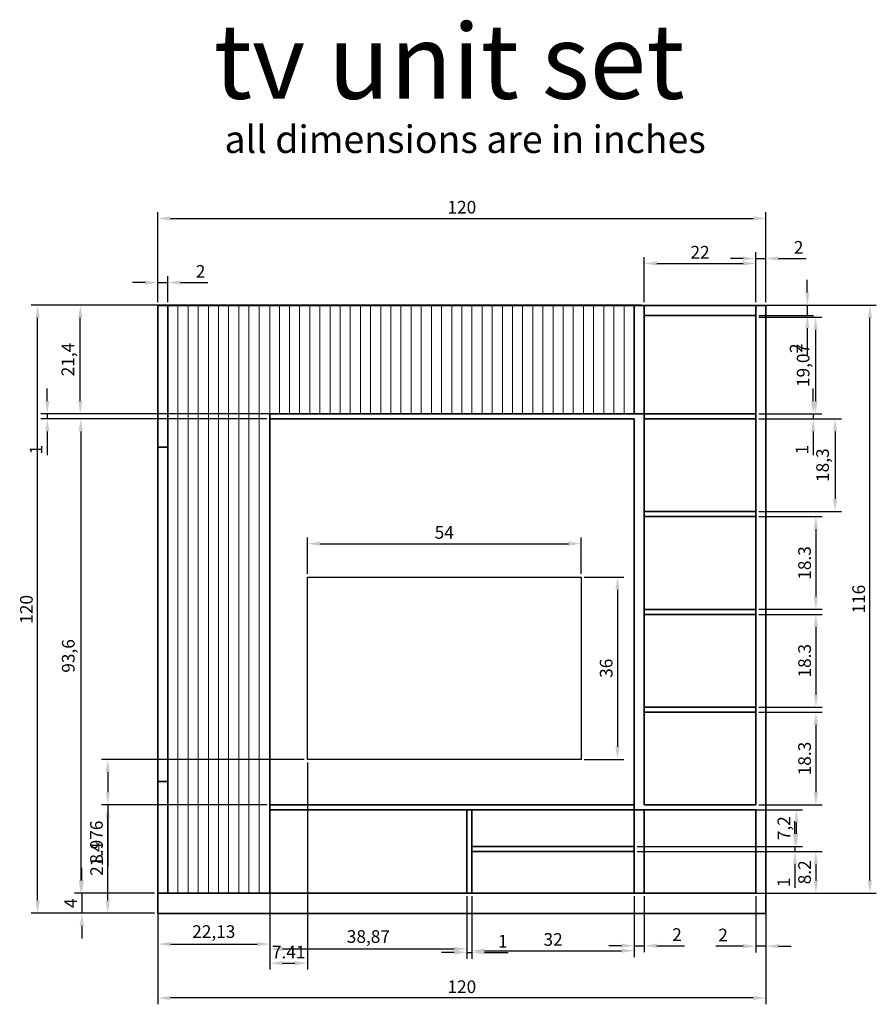
# Model space of a CAD drawing. Units: inches. Extents: x 64 to 1096, y 24 to 3074.
# Tile 1 of 1: x 64.3 to 233.3, y 23.5 to 217.9. Entities that reach past the tile are written whole.
import ezdxf

# ---------------------------------------------------------------- set-up
doc = ezdxf.new("R2010")
doc.units = ezdxf.units.IN
for name, color, linetype, lineweight in [('A-ANNO-DIMS', 2, 'Continuous', 18), ('A-ANNO-TEXT', 3, 'Continuous', 25), ('A-EQPM', 4, 'Continuous', 25), ('A-FURN', 7, 'Continuous', 35), ('A-FURN-PATT', 8, 'Continuous', 13)]:
    doc.layers.add(name, color=color, linetype=linetype, lineweight=lineweight)
doc.styles.get("Standard").update_dxf_attribs({"font": 'arial.ttf'})
doc.dimstyles.new('ISO-25', dxfattribs={"dimtxt": 2.5, "dimasz": 2.5, "dimexe": 1.25, "dimexo": 0.625, "dimtad": 1, "dimtxsty": 'Standard', "dimcen": 2.5, "dimadec": 0, "dimazin": 0, "dimtfac": 1, "dimtmove": 0, "dimatfit": 3, "dimfxl": 1, "dimarcsym": 0})

# ---------------------------------------------------------------- blocks, each defined once
blk = doc.blocks.new('*D1')
at = {"layer": 'A-ANNO-DIMS', "color": 0, "lineweight": -2, "transparency": 16777216}
for p, q in [((219.69, 163.98), (219.69, 166.48)), ((210.15, 161.48), (220.94, 161.48)), ((219.69, 161.48), (219.69, 159.48)), ((210.15, 159.48), (220.94, 159.48)), ((219.69, 156.98), (219.69, 151.57))]:
    blk.add_line(p, q, dxfattribs=at)
at = {"layer": 'A-ANNO-DIMS', "color": 0, "transparency": 16777216}
for points in [[(219.28, 163.98), (220.11, 163.98), (219.69, 161.48)], [(219.28, 156.98), (220.11, 156.98), (219.69, 159.48)]]:
    blk.add_solid(points, dxfattribs=at)
at = {"layer": 'Defpoints', "color": 0, "transparency": 16777216}
for p in [(209.53, 161.48), (209.53, 159.48), (219.69, 159.48)]:
    blk.add_point(p, dxfattribs=at)
at = {"layer": 'A-ANNO-DIMS', "color": 0, "transparency": 16777216, "insert": (217.81, 153.02), "char_height": 2.5, "attachment_point": 5, "rotation": 90}
blk.add_mtext('2', dxfattribs=at)
blk = doc.blocks.new('*D2')
at = {"layer": 'A-ANNO-DIMS', "color": 0, "lineweight": -2, "transparency": 16777216}
for p, q in [((210.15, 159.15), (222.57, 159.15)), ((221.32, 156.65), (221.32, 142.58)), ((210.15, 140.08), (222.57, 140.08))]:
    blk.add_line(p, q, dxfattribs=at)
at = {"layer": 'A-ANNO-DIMS', "color": 0, "transparency": 16777216}
for points in [[(220.9, 156.65), (221.73, 156.65), (221.32, 159.15)], [(220.9, 142.58), (221.73, 142.58), (221.32, 140.08)]]:
    blk.add_solid(points, dxfattribs=at)
at = {"layer": 'Defpoints', "color": 0, "transparency": 16777216}
for p in [(209.53, 159.15), (209.53, 140.08), (221.32, 140.08)]:
    blk.add_point(p, dxfattribs=at)
at = {"layer": 'A-ANNO-DIMS', "color": 0, "transparency": 16777216, "insert": (219.19, 149.61), "char_height": 2.5, "attachment_point": 5, "rotation": 90}
blk.add_mtext('19,07', dxfattribs=at)
blk = doc.blocks.new('*D3')
at = {"layer": 'A-ANNO-DIMS', "color": 0, "lineweight": -2, "transparency": 16777216}
for p, q in [((220.85, 142.58), (220.85, 145.08)), ((210.15, 140.08), (222.1, 140.08)), ((220.85, 140.08), (220.85, 139.08)), ((210.15, 139.08), (222.1, 139.08)), ((220.85, 136.58), (220.85, 131.91))]:
    blk.add_line(p, q, dxfattribs=at)
at = {"layer": 'A-ANNO-DIMS', "color": 0, "transparency": 16777216}
for points in [[(220.43, 142.58), (221.26, 142.58), (220.85, 140.08)], [(220.43, 136.58), (221.26, 136.58), (220.85, 139.08)]]:
    blk.add_solid(points, dxfattribs=at)
at = {"layer": 'Defpoints', "color": 0, "transparency": 16777216}
for p in [(209.53, 140.08), (209.53, 139.08), (220.85, 139.08)]:
    blk.add_point(p, dxfattribs=at)
at = {"layer": 'A-ANNO-DIMS', "color": 0, "transparency": 16777216, "insert": (218.97, 132.99), "char_height": 2.5, "attachment_point": 5, "rotation": 90}
blk.add_mtext('1', dxfattribs=at)
blk = doc.blocks.new('*D4')
at = {"layer": 'A-ANNO-DIMS', "color": 0, "lineweight": -2, "transparency": 16777216}
for p, q in [((210.15, 139.08), (226.41, 139.08)), ((225.16, 136.58), (225.16, 123.28)), ((210.15, 120.78), (226.41, 120.78))]:
    blk.add_line(p, q, dxfattribs=at)
at = {"layer": 'A-ANNO-DIMS', "color": 0, "transparency": 16777216}
for points in [[(224.74, 136.58), (225.58, 136.58), (225.16, 139.08)], [(224.74, 123.28), (225.58, 123.28), (225.16, 120.78)]]:
    blk.add_solid(points, dxfattribs=at)
at = {"layer": 'Defpoints', "color": 0, "transparency": 16777216}
for p in [(209.53, 139.08), (209.53, 120.78), (225.16, 120.78)]:
    blk.add_point(p, dxfattribs=at)
at = {"layer": 'A-ANNO-DIMS', "color": 0, "transparency": 16777216, "insert": (223.03, 129.93), "char_height": 2.5, "attachment_point": 5, "rotation": 90}
blk.add_mtext('18,3', dxfattribs=at)
blk = doc.blocks.new('*D5')
at = {"layer": 'A-ANNO-DIMS', "color": 0, "lineweight": -2, "transparency": 16777216}
for p, q in [((187.53, 162.1), (187.53, 171)), ((190.03, 169.75), (207.03, 169.75)), ((209.53, 162.1), (209.53, 171))]:
    blk.add_line(p, q, dxfattribs=at)
at = {"layer": 'A-ANNO-DIMS', "color": 0, "transparency": 16777216}
for points in [[(190.03, 170.17), (190.03, 169.33), (187.53, 169.75)], [(207.03, 170.17), (207.03, 169.33), (209.53, 169.75)]]:
    blk.add_solid(points, dxfattribs=at)
at = {"layer": 'Defpoints', "color": 0, "transparency": 16777216}
for p in [(209.53, 169.75), (187.53, 161.48), (209.53, 161.48)]:
    blk.add_point(p, dxfattribs=at)
at = {"layer": 'A-ANNO-DIMS', "color": 0, "transparency": 16777216, "insert": (198.53, 171.63), "char_height": 2.5, "attachment_point": 5}
blk.add_mtext('22', dxfattribs=at)
blk = doc.blocks.new('*D6')
at = {"layer": 'A-ANNO-DIMS', "color": 0, "lineweight": -2, "transparency": 16777216}
for p, q in [((209.53, 162.1), (209.53, 171.97)), ((211.53, 162.1), (211.53, 171.97)), ((207.03, 170.72), (204.53, 170.72)), ((209.53, 170.72), (211.53, 170.72)), ((214.03, 170.72), (219.43, 170.72))]:
    blk.add_line(p, q, dxfattribs=at)
at = {"layer": 'A-ANNO-DIMS', "color": 0, "transparency": 16777216}
for points in [[(207.03, 171.13), (207.03, 170.3), (209.53, 170.72)], [(214.03, 171.13), (214.03, 170.3), (211.53, 170.72)]]:
    blk.add_solid(points, dxfattribs=at)
at = {"layer": 'Defpoints', "color": 0, "transparency": 16777216}
for p in [(211.53, 170.72), (209.53, 161.48), (211.53, 161.48)]:
    blk.add_point(p, dxfattribs=at)
at = {"layer": 'A-ANNO-DIMS', "color": 0, "transparency": 16777216, "insert": (217.98, 172.6), "char_height": 2.5, "attachment_point": 5}
blk.add_mtext('2', dxfattribs=at)
blk = doc.blocks.new('*D7')
at = {"layer": 'A-ANNO-DIMS', "color": 0, "lineweight": -2, "transparency": 16777216}
for p, q in [((212.15, 161.48), (233.3, 161.48)), ((232.05, 47.98), (232.05, 158.98)), ((210.15, 45.48), (233.3, 45.48))]:
    blk.add_line(p, q, dxfattribs=at)
at = {"layer": 'A-ANNO-DIMS', "color": 0, "transparency": 16777216}
for points in [[(231.63, 158.98), (232.47, 158.98), (232.05, 161.48)], [(231.63, 47.98), (232.47, 47.98), (232.05, 45.48)]]:
    blk.add_solid(points, dxfattribs=at)
at = {"layer": 'Defpoints', "color": 0, "transparency": 16777216}
for p in [(211.53, 161.48), (232.05, 161.48), (209.53, 45.48)]:
    blk.add_point(p, dxfattribs=at)
at = {"layer": 'A-ANNO-DIMS', "color": 0, "transparency": 16777216, "insert": (230.15, 103.48), "char_height": 2.5, "attachment_point": 5, "rotation": 90}
blk.add_mtext('116', dxfattribs=at)
blk = doc.blocks.new('*D8')
at = {"layer": 'A-ANNO-DIMS', "color": 0, "lineweight": -2, "transparency": 16777216}
for p, q in [((91.53, 162.1), (91.53, 167.23)), ((93.53, 162.1), (93.53, 167.23)), ((89.03, 165.98), (86.53, 165.98)), ((91.53, 165.98), (93.53, 165.98)), ((96.03, 165.98), (101.43, 165.98))]:
    blk.add_line(p, q, dxfattribs=at)
at = {"layer": 'A-ANNO-DIMS', "color": 0, "transparency": 16777216}
for points in [[(89.03, 166.39), (89.03, 165.56), (91.53, 165.98)], [(96.03, 166.39), (96.03, 165.56), (93.53, 165.98)]]:
    blk.add_solid(points, dxfattribs=at)
at = {"layer": 'Defpoints', "color": 0, "transparency": 16777216}
for p in [(93.53, 165.98), (91.53, 161.48), (93.53, 161.48)]:
    blk.add_point(p, dxfattribs=at)
at = {"layer": 'A-ANNO-DIMS', "color": 0, "transparency": 16777216, "insert": (99.98, 167.86), "char_height": 2.5, "attachment_point": 5}
blk.add_mtext('2', dxfattribs=at)
blk = doc.blocks.new('*D9')
at = {"layer": 'A-ANNO-DIMS', "color": 0, "lineweight": -2, "transparency": 16777216}
for p, q in [((91.53, 162.1), (91.53, 179.88)), ((211.53, 162.1), (211.53, 179.88)), ((94.03, 178.63), (209.03, 178.63))]:
    blk.add_line(p, q, dxfattribs=at)
at = {"layer": 'A-ANNO-DIMS', "color": 0, "transparency": 16777216}
for points in [[(94.03, 179.05), (94.03, 178.21), (91.53, 178.63)], [(209.03, 179.05), (209.03, 178.21), (211.53, 178.63)]]:
    blk.add_solid(points, dxfattribs=at)
at = {"layer": 'Defpoints', "color": 0, "transparency": 16777216}
for p in [(211.53, 178.63), (91.53, 161.48), (211.53, 161.48)]:
    blk.add_point(p, dxfattribs=at)
at = {"layer": 'A-ANNO-DIMS', "color": 0, "transparency": 16777216, "insert": (151.53, 180.53), "char_height": 2.5, "attachment_point": 5}
blk.add_mtext('120', dxfattribs=at)
blk = doc.blocks.new('*D10')
at = {"layer": 'A-ANNO-DIMS', "color": 0, "lineweight": -2, "transparency": 16777216}
for p, q in [((186.9, 161.48), (75, 161.48)), ((76.25, 142.58), (76.25, 158.98)), ((186.9, 140.08), (75, 140.08))]:
    blk.add_line(p, q, dxfattribs=at)
at = {"layer": 'A-ANNO-DIMS', "color": 0, "transparency": 16777216}
for points in [[(75.83, 158.98), (76.66, 158.98), (76.25, 161.48)], [(75.83, 142.58), (76.66, 142.58), (76.25, 140.08)]]:
    blk.add_solid(points, dxfattribs=at)
at = {"layer": 'Defpoints', "color": 0, "transparency": 16777216}
for p in [(76.25, 161.48), (187.53, 161.48), (187.53, 140.08)]:
    blk.add_point(p, dxfattribs=at)
at = {"layer": 'A-ANNO-DIMS', "color": 0, "transparency": 16777216, "insert": (74.12, 150.78), "char_height": 2.5, "attachment_point": 5, "rotation": 90}
blk.add_mtext('21,4', dxfattribs=at)
blk = doc.blocks.new('*D11')
at = {"layer": 'A-ANNO-DIMS', "color": 0, "lineweight": -2, "transparency": 16777216}
for p, q in [((90.9, 139.08), (75.09, 139.08)), ((76.34, 136.58), (76.34, 47.98)), ((90.9, 45.48), (75.09, 45.48))]:
    blk.add_line(p, q, dxfattribs=at)
at = {"layer": 'A-ANNO-DIMS', "color": 0, "transparency": 16777216}
for points in [[(75.92, 136.58), (76.76, 136.58), (76.34, 139.08)], [(75.92, 47.98), (76.76, 47.98), (76.34, 45.48)]]:
    blk.add_solid(points, dxfattribs=at)
at = {"layer": 'Defpoints', "color": 0, "transparency": 16777216}
for p in [(91.53, 139.08), (76.34, 45.48), (91.53, 45.48)]:
    blk.add_point(p, dxfattribs=at)
at = {"layer": 'A-ANNO-DIMS', "color": 0, "transparency": 16777216, "insert": (74.21, 92.28), "char_height": 2.5, "attachment_point": 5, "rotation": 90}
blk.add_mtext('93,6', dxfattribs=at)
blk = doc.blocks.new('*D12')
at = {"layer": 'A-ANNO-DIMS', "color": 0, "lineweight": -2, "transparency": 16777216}
for p, q in [((69.74, 142.58), (69.74, 145.08)), ((113.03, 140.08), (68.49, 140.08)), ((69.74, 140.08), (69.74, 139.08)), ((113.03, 139.08), (68.49, 139.08)), ((69.74, 136.58), (69.74, 131.91))]:
    blk.add_line(p, q, dxfattribs=at)
at = {"layer": 'A-ANNO-DIMS', "color": 0, "transparency": 16777216}
for points in [[(69.33, 142.58), (70.16, 142.58), (69.74, 140.08)], [(69.33, 136.58), (70.16, 136.58), (69.74, 139.08)]]:
    blk.add_solid(points, dxfattribs=at)
at = {"layer": 'Defpoints', "color": 0, "transparency": 16777216}
for p in [(113.65, 140.08), (69.74, 139.08), (113.65, 139.08)]:
    blk.add_point(p, dxfattribs=at)
at = {"layer": 'A-ANNO-DIMS', "color": 0, "transparency": 16777216, "insert": (67.86, 132.99), "char_height": 2.5, "attachment_point": 5, "rotation": 90}
blk.add_mtext('1', dxfattribs=at)
blk = doc.blocks.new('*D13')
at = {"layer": 'A-ANNO-DIMS', "color": 0, "lineweight": -2, "transparency": 16777216}
for p, q in [((76.56, 47.98), (76.56, 50.48)), ((90.9, 45.48), (75.31, 45.48)), ((76.56, 45.48), (76.56, 41.48)), ((90.9, 41.48), (75.31, 41.48)), ((76.56, 38.98), (76.56, 36.48))]:
    blk.add_line(p, q, dxfattribs=at)
at = {"layer": 'A-ANNO-DIMS', "color": 0, "transparency": 16777216}
for points in [[(76.14, 47.98), (76.97, 47.98), (76.56, 45.48)], [(76.14, 38.98), (76.97, 38.98), (76.56, 41.48)]]:
    blk.add_solid(points, dxfattribs=at)
at = {"layer": 'Defpoints', "color": 0, "transparency": 16777216}
for p in [(91.53, 45.48), (76.56, 41.48), (91.53, 41.48)]:
    blk.add_point(p, dxfattribs=at)
at = {"layer": 'A-ANNO-DIMS', "color": 0, "transparency": 16777216, "insert": (74.68, 43.48), "char_height": 2.5, "attachment_point": 5, "rotation": 90}
blk.add_mtext('4', dxfattribs=at)
blk = doc.blocks.new('*D14')
at = {"layer": 'A-ANNO-DIMS', "color": 0, "lineweight": -2, "transparency": 16777216}
for p, q in [((90.9, 161.48), (66.59, 161.48)), ((67.84, 43.98), (67.84, 158.98)), ((90.9, 41.48), (66.59, 41.48))]:
    blk.add_line(p, q, dxfattribs=at)
at = {"layer": 'A-ANNO-DIMS', "color": 0, "transparency": 16777216}
for points in [[(67.42, 158.98), (68.26, 158.98), (67.84, 161.48)], [(67.42, 43.98), (68.26, 43.98), (67.84, 41.48)]]:
    blk.add_solid(points, dxfattribs=at)
at = {"layer": 'Defpoints', "color": 0, "transparency": 16777216}
for p in [(67.84, 161.48), (91.53, 161.48), (91.53, 41.48)]:
    blk.add_point(p, dxfattribs=at)
at = {"layer": 'A-ANNO-DIMS', "color": 0, "transparency": 16777216, "insert": (65.94, 101.48), "char_height": 2.5, "attachment_point": 5, "rotation": 90}
blk.add_mtext('120', dxfattribs=at)
blk = doc.blocks.new('*D15')
at = {"layer": 'A-ANNO-DIMS', "color": 0, "lineweight": -2, "transparency": 16777216}
for p, q in [((91.53, 44.85), (91.53, 34.17)), ((113.65, 44.85), (113.65, 34.17)), ((94.03, 35.42), (111.15, 35.42))]:
    blk.add_line(p, q, dxfattribs=at)
at = {"layer": 'A-ANNO-DIMS', "color": 0, "transparency": 16777216}
for points in [[(94.03, 35.83), (94.03, 35), (91.53, 35.42)], [(111.15, 35.83), (111.15, 35), (113.65, 35.42)]]:
    blk.add_solid(points, dxfattribs=at)
at = {"layer": 'Defpoints', "color": 0, "transparency": 16777216}
for p in [(91.53, 45.48), (113.65, 45.48), (113.65, 35.42)]:
    blk.add_point(p, dxfattribs=at)
at = {"layer": 'A-ANNO-DIMS', "color": 0, "transparency": 16777216, "insert": (102.59, 37.55), "char_height": 2.5, "attachment_point": 5}
blk.add_mtext('22,13', dxfattribs=at)
blk = doc.blocks.new('*D16')
at = {"layer": 'A-ANNO-DIMS', "color": 0, "lineweight": -2, "transparency": 16777216}
for p, q in [((113.65, 44.85), (113.65, 33.2)), ((152.53, 44.85), (152.53, 33.2)), ((116.15, 34.45), (150.03, 34.45))]:
    blk.add_line(p, q, dxfattribs=at)
at = {"layer": 'A-ANNO-DIMS', "color": 0, "transparency": 16777216}
for points in [[(116.15, 34.87), (116.15, 34.03), (113.65, 34.45)], [(150.03, 34.87), (150.03, 34.03), (152.53, 34.45)]]:
    blk.add_solid(points, dxfattribs=at)
at = {"layer": 'Defpoints', "color": 0, "transparency": 16777216}
for p in [(113.65, 45.48), (152.53, 45.48), (152.53, 34.45)]:
    blk.add_point(p, dxfattribs=at)
at = {"layer": 'A-ANNO-DIMS', "color": 0, "transparency": 16777216, "insert": (133.09, 36.58), "char_height": 2.5, "attachment_point": 5}
blk.add_mtext('38,87', dxfattribs=at)
blk = doc.blocks.new('*D17')
at = {"layer": 'A-ANNO-DIMS', "color": 0, "lineweight": -2, "transparency": 16777216}
for p, q in [((152.53, 44.85), (152.53, 32.53)), ((153.53, 44.85), (153.53, 32.53)), ((150.03, 33.78), (147.53, 33.78)), ((152.53, 33.78), (153.53, 33.78)), ((156.03, 33.78), (160.7, 33.78))]:
    blk.add_line(p, q, dxfattribs=at)
at = {"layer": 'A-ANNO-DIMS', "color": 0, "transparency": 16777216}
for points in [[(150.03, 34.2), (150.03, 33.36), (152.53, 33.78)], [(156.03, 34.2), (156.03, 33.36), (153.53, 33.78)]]:
    blk.add_solid(points, dxfattribs=at)
at = {"layer": 'Defpoints', "color": 0, "transparency": 16777216}
for p in [(152.53, 45.48), (153.53, 45.48), (153.53, 33.78)]:
    blk.add_point(p, dxfattribs=at)
at = {"layer": 'A-ANNO-DIMS', "color": 0, "transparency": 16777216, "insert": (159.61, 35.66), "char_height": 2.5, "attachment_point": 5}
blk.add_mtext('1', dxfattribs=at)
blk = doc.blocks.new('*D18')
at = {"layer": 'A-ANNO-DIMS', "color": 0, "lineweight": -2, "transparency": 16777216}
for p, q in [((153.53, 44.85), (153.53, 32.85)), ((185.53, 44.85), (185.53, 32.85)), ((156.03, 34.1), (183.03, 34.1))]:
    blk.add_line(p, q, dxfattribs=at)
at = {"layer": 'A-ANNO-DIMS', "color": 0, "transparency": 16777216}
for points in [[(156.03, 34.52), (156.03, 33.68), (153.53, 34.1)], [(183.03, 34.52), (183.03, 33.68), (185.53, 34.1)]]:
    blk.add_solid(points, dxfattribs=at)
at = {"layer": 'Defpoints', "color": 0, "transparency": 16777216}
for p in [(153.53, 45.48), (185.53, 45.48), (185.53, 34.1)]:
    blk.add_point(p, dxfattribs=at)
at = {"layer": 'A-ANNO-DIMS', "color": 0, "transparency": 16777216, "insert": (169.53, 36), "char_height": 2.5, "attachment_point": 5}
blk.add_mtext('32', dxfattribs=at)
blk = doc.blocks.new('*D19')
at = {"layer": 'A-ANNO-DIMS', "color": 0, "lineweight": -2, "transparency": 16777216}
for p, q in [((185.53, 44.85), (185.53, 33.83)), ((187.53, 44.85), (187.53, 33.83)), ((183.03, 35.08), (180.53, 35.08)), ((185.53, 35.08), (187.53, 35.08)), ((190.03, 35.08), (195.43, 35.08))]:
    blk.add_line(p, q, dxfattribs=at)
at = {"layer": 'A-ANNO-DIMS', "color": 0, "transparency": 16777216}
for points in [[(183.03, 35.5), (183.03, 34.66), (185.53, 35.08)], [(190.03, 35.5), (190.03, 34.66), (187.53, 35.08)]]:
    blk.add_solid(points, dxfattribs=at)
at = {"layer": 'Defpoints', "color": 0, "transparency": 16777216}
for p in [(185.53, 45.48), (187.53, 45.48), (187.53, 35.08)]:
    blk.add_point(p, dxfattribs=at)
at = {"layer": 'A-ANNO-DIMS', "color": 0, "transparency": 16777216, "insert": (193.98, 36.96), "char_height": 2.5, "attachment_point": 5}
blk.add_mtext('2', dxfattribs=at)
blk = doc.blocks.new('*D20')
at = {"layer": 'A-ANNO-DIMS', "color": 0, "lineweight": -2, "transparency": 16777216}
for p, q in [((209.53, 44.85), (209.53, 33.75)), ((211.53, 44.85), (211.53, 33.75)), ((207.03, 35), (201.62, 35)), ((211.53, 35), (209.53, 35)), ((214.03, 35), (216.53, 35))]:
    blk.add_line(p, q, dxfattribs=at)
at = {"layer": 'A-ANNO-DIMS', "color": 0, "transparency": 16777216}
for points in [[(207.03, 35.41), (207.03, 34.58), (209.53, 35)], [(214.03, 35.41), (214.03, 34.58), (211.53, 35)]]:
    blk.add_solid(points, dxfattribs=at)
at = {"layer": 'Defpoints', "color": 0, "transparency": 16777216}
for p in [(209.53, 45.48), (211.53, 45.48), (209.53, 35)]:
    blk.add_point(p, dxfattribs=at)
at = {"layer": 'A-ANNO-DIMS', "color": 0, "transparency": 16777216, "insert": (203.07, 36.88), "char_height": 2.5, "attachment_point": 5}
blk.add_mtext('2', dxfattribs=at)
blk = doc.blocks.new('*D21')
at = {"layer": 'A-ANNO-DIMS', "color": 0, "lineweight": -2, "transparency": 16777216}
for p, q in [((91.53, 44.85), (91.53, 23.52)), ((211.53, 44.85), (211.53, 23.52)), ((209.03, 24.77), (94.03, 24.77))]:
    blk.add_line(p, q, dxfattribs=at)
at = {"layer": 'A-ANNO-DIMS', "color": 0, "transparency": 16777216}
for points in [[(94.03, 25.19), (94.03, 24.36), (91.53, 24.77)], [(209.03, 25.19), (209.03, 24.36), (211.53, 24.77)]]:
    blk.add_solid(points, dxfattribs=at)
at = {"layer": 'Defpoints', "color": 0, "transparency": 16777216}
for p in [(91.53, 45.48), (211.53, 45.48), (91.53, 24.77)]:
    blk.add_point(p, dxfattribs=at)
at = {"layer": 'A-ANNO-DIMS', "color": 0, "transparency": 16777216, "insert": (151.53, 26.67), "char_height": 2.5, "attachment_point": 5}
blk.add_mtext('120', dxfattribs=at)
blk = doc.blocks.new('*D22')
at = {"layer": 'A-ANNO-DIMS', "color": 0, "lineweight": -2, "transparency": 16777216}
for p, q in [((186.15, 61.88), (218.77, 61.88)), ((217.52, 59.38), (217.52, 57.18)), ((186.15, 54.68), (218.77, 54.68))]:
    blk.add_line(p, q, dxfattribs=at)
at = {"layer": 'A-ANNO-DIMS', "color": 0, "transparency": 16777216}
for points in [[(217.1, 59.38), (217.94, 59.38), (217.52, 61.88)], [(217.1, 57.18), (217.94, 57.18), (217.52, 54.68)]]:
    blk.add_solid(points, dxfattribs=at)
at = {"layer": 'Defpoints', "color": 0, "transparency": 16777216}
for p in [(185.53, 61.88), (185.53, 54.68), (217.52, 54.68)]:
    blk.add_point(p, dxfattribs=at)
at = {"layer": 'A-ANNO-DIMS', "color": 0, "transparency": 16777216, "insert": (215.39, 58.28), "char_height": 2.5, "attachment_point": 5, "rotation": 90}
blk.add_mtext('7,2', dxfattribs=at)
blk = doc.blocks.new('*D23')
at = {"layer": 'A-ANNO-DIMS', "color": 0, "lineweight": -2, "transparency": 16777216}
for p, q in [((217.25, 57.18), (217.25, 59.68)), ((186.15, 54.68), (218.5, 54.68)), ((217.25, 54.68), (217.25, 53.68)), ((186.15, 53.68), (218.5, 53.68)), ((217.25, 51.18), (217.25, 46.51))]:
    blk.add_line(p, q, dxfattribs=at)
at = {"layer": 'A-ANNO-DIMS', "color": 0, "transparency": 16777216}
for points in [[(216.84, 57.18), (217.67, 57.18), (217.25, 54.68)], [(216.84, 51.18), (217.67, 51.18), (217.25, 53.68)]]:
    blk.add_solid(points, dxfattribs=at)
at = {"layer": 'Defpoints', "color": 0, "transparency": 16777216}
for p in [(185.53, 54.68), (185.53, 53.68), (217.25, 53.68)]:
    blk.add_point(p, dxfattribs=at)
at = {"layer": 'A-ANNO-DIMS', "color": 0, "transparency": 16777216, "insert": (215.37, 47.59), "char_height": 2.5, "attachment_point": 5, "rotation": 90}
blk.add_mtext('1', dxfattribs=at)
blk = doc.blocks.new('*D24')
at = {"layer": 'A-ANNO-DIMS', "color": 0, "lineweight": -2, "transparency": 16777216}
for p, q in [((175.69, 107.85), (183.49, 107.85)), ((182.24, 105.35), (182.24, 74.35)), ((175.69, 71.85), (183.49, 71.85))]:
    blk.add_line(p, q, dxfattribs=at)
at = {"layer": 'A-ANNO-DIMS', "color": 0, "transparency": 16777216}
for points in [[(181.82, 105.35), (182.65, 105.35), (182.24, 107.85)], [(181.82, 74.35), (182.65, 74.35), (182.24, 71.85)]]:
    blk.add_solid(points, dxfattribs=at)
at = {"layer": 'Defpoints', "color": 0, "transparency": 16777216}
for p in [(175.06, 107.85), (175.06, 71.85), (182.24, 71.85)]:
    blk.add_point(p, dxfattribs=at)
at = {"layer": 'A-ANNO-DIMS', "color": 0, "transparency": 16777216, "insert": (180.33, 89.85), "char_height": 2.5, "attachment_point": 5, "rotation": 90}
blk.add_mtext('36', dxfattribs=at)
blk = doc.blocks.new('*D25')
at = {"layer": 'A-ANNO-DIMS', "color": 0, "lineweight": -2, "transparency": 16777216}
for p, q in [((121.06, 108.48), (121.06, 115.69)), ((175.06, 108.48), (175.06, 115.69)), ((123.56, 114.44), (172.56, 114.44))]:
    blk.add_line(p, q, dxfattribs=at)
at = {"layer": 'A-ANNO-DIMS', "color": 0, "transparency": 16777216}
for points in [[(123.56, 114.86), (123.56, 114.02), (121.06, 114.44)], [(172.56, 114.86), (172.56, 114.02), (175.06, 114.44)]]:
    blk.add_solid(points, dxfattribs=at)
at = {"layer": 'Defpoints', "color": 0, "transparency": 16777216}
for p in [(175.06, 114.44), (121.06, 107.85), (175.06, 107.85)]:
    blk.add_point(p, dxfattribs=at)
at = {"layer": 'A-ANNO-DIMS', "color": 0, "transparency": 16777216, "insert": (148.06, 116.34), "char_height": 2.5, "attachment_point": 5}
blk.add_mtext('54', dxfattribs=at)
blk = doc.blocks.new('*D26')
at = {"layer": 'A-ANNO-DIMS', "color": 0, "lineweight": -2, "transparency": 16777216}
for p, q in [((210.15, 119.78), (222.63, 119.78)), ((221.38, 117.28), (221.38, 103.98)), ((210.15, 101.48), (222.63, 101.48))]:
    blk.add_line(p, q, dxfattribs=at)
at = {"layer": 'A-ANNO-DIMS', "color": 0, "transparency": 16777216}
for points in [[(220.96, 117.28), (221.79, 117.28), (221.38, 119.78)], [(220.96, 103.98), (221.79, 103.98), (221.38, 101.48)]]:
    blk.add_solid(points, dxfattribs=at)
at = {"layer": 'Defpoints', "color": 0, "transparency": 16777216}
for p in [(209.53, 119.78), (209.53, 101.48), (221.38, 101.48)]:
    blk.add_point(p, dxfattribs=at)
at = {"layer": 'A-ANNO-DIMS', "color": 0, "transparency": 16777216, "insert": (219.47, 110.63), "char_height": 2.5, "attachment_point": 5, "rotation": 90}
blk.add_mtext('18.3', dxfattribs=at)
blk = doc.blocks.new('*D27')
at = {"layer": 'A-ANNO-DIMS', "color": 0, "lineweight": -2, "transparency": 16777216}
for p, q in [((210.15, 100.48), (222.63, 100.48)), ((221.38, 97.98), (221.38, 84.68)), ((210.15, 82.18), (222.63, 82.18))]:
    blk.add_line(p, q, dxfattribs=at)
at = {"layer": 'A-ANNO-DIMS', "color": 0, "transparency": 16777216}
for points in [[(220.96, 97.98), (221.79, 97.98), (221.38, 100.48)], [(220.96, 84.68), (221.79, 84.68), (221.38, 82.18)]]:
    blk.add_solid(points, dxfattribs=at)
at = {"layer": 'Defpoints', "color": 0, "transparency": 16777216}
for p in [(209.53, 100.48), (209.53, 82.18), (221.38, 82.18)]:
    blk.add_point(p, dxfattribs=at)
at = {"layer": 'A-ANNO-DIMS', "color": 0, "transparency": 16777216, "insert": (219.47, 91.33), "char_height": 2.5, "attachment_point": 5, "rotation": 90}
blk.add_mtext('18.3', dxfattribs=at)
blk = doc.blocks.new('*D28')
at = {"layer": 'A-ANNO-DIMS', "color": 0, "lineweight": -2, "transparency": 16777216}
for p, q in [((210.15, 81.18), (222.63, 81.18)), ((221.38, 78.68), (221.38, 65.38)), ((210.15, 62.88), (222.63, 62.88))]:
    blk.add_line(p, q, dxfattribs=at)
at = {"layer": 'A-ANNO-DIMS', "color": 0, "transparency": 16777216}
for points in [[(220.96, 78.68), (221.79, 78.68), (221.38, 81.18)], [(220.96, 65.38), (221.79, 65.38), (221.38, 62.88)]]:
    blk.add_solid(points, dxfattribs=at)
at = {"layer": 'Defpoints', "color": 0, "transparency": 16777216}
for p in [(209.53, 81.18), (209.53, 62.88), (221.38, 62.88)]:
    blk.add_point(p, dxfattribs=at)
at = {"layer": 'A-ANNO-DIMS', "color": 0, "transparency": 16777216, "insert": (219.47, 72.03), "char_height": 2.5, "attachment_point": 5, "rotation": 90}
blk.add_mtext('18.3', dxfattribs=at)
blk = doc.blocks.new('*D29')
at = {"layer": 'A-ANNO-DIMS', "color": 0, "lineweight": -2, "transparency": 16777216}
for p, q in [((121.06, 71.23), (121.06, 30.38)), ((113.65, 62.25), (113.65, 30.38)), ((116.15, 31.63), (118.56, 31.63))]:
    blk.add_line(p, q, dxfattribs=at)
at = {"layer": 'A-ANNO-DIMS', "color": 0, "transparency": 16777216}
for points in [[(116.15, 32.04), (116.15, 31.21), (113.65, 31.63)], [(118.56, 32.04), (118.56, 31.21), (121.06, 31.63)]]:
    blk.add_solid(points, dxfattribs=at)
at = {"layer": 'Defpoints', "color": 0, "transparency": 16777216}
for p in [(121.06, 71.85), (113.65, 62.88), (121.06, 31.63)]:
    blk.add_point(p, dxfattribs=at)
at = {"layer": 'A-ANNO-DIMS', "color": 0, "transparency": 16777216, "insert": (117.36, 33.51), "char_height": 2.5, "attachment_point": 5}
blk.add_mtext('7.41', dxfattribs=at)
blk = doc.blocks.new('*D30')
at = {"layer": 'A-ANNO-DIMS', "color": 0, "lineweight": -2, "transparency": 16777216}
for p, q in [((120.44, 71.85), (80.43, 71.85)), ((81.68, 69.35), (81.68, 65.38)), ((113.03, 62.88), (80.43, 62.88)), ((81.68, 62.88), (81.68, 50.69))]:
    blk.add_line(p, q, dxfattribs=at)
at = {"layer": 'A-ANNO-DIMS', "color": 0, "transparency": 16777216}
for points in [[(81.26, 69.35), (82.09, 69.35), (81.68, 71.85)], [(81.26, 65.38), (82.09, 65.38), (81.68, 62.88)]]:
    blk.add_solid(points, dxfattribs=at)
at = {"layer": 'Defpoints', "color": 0, "transparency": 16777216}
for p in [(121.06, 71.85), (81.68, 62.88), (113.65, 62.88)]:
    blk.add_point(p, dxfattribs=at)
at = {"layer": 'A-ANNO-DIMS', "color": 0, "transparency": 16777216, "insert": (79.77, 55.53), "char_height": 2.5, "attachment_point": 5, "rotation": 90}
blk.add_mtext('8.976', dxfattribs=at)
blk = doc.blocks.new('*D31')
at = {"layer": 'A-ANNO-DIMS', "color": 0, "lineweight": -2, "transparency": 16777216}
for p, q in [((186.15, 53.68), (222.63, 53.68)), ((221.38, 51.18), (221.38, 47.98)), ((186.15, 45.48), (222.63, 45.48))]:
    blk.add_line(p, q, dxfattribs=at)
at = {"layer": 'A-ANNO-DIMS', "color": 0, "transparency": 16777216}
for points in [[(220.96, 51.18), (221.79, 51.18), (221.38, 53.68)], [(220.96, 47.98), (221.79, 47.98), (221.38, 45.48)]]:
    blk.add_solid(points, dxfattribs=at)
at = {"layer": 'Defpoints', "color": 0, "transparency": 16777216}
for p in [(185.53, 53.68), (185.53, 45.48), (221.38, 45.48)]:
    blk.add_point(p, dxfattribs=at)
at = {"layer": 'A-ANNO-DIMS', "color": 0, "transparency": 16777216, "insert": (219.47, 49.58), "char_height": 2.5, "attachment_point": 5, "rotation": 90}
blk.add_mtext('8.2', dxfattribs=at)
blk = doc.blocks.new('*D32')
at = {"layer": 'A-ANNO-DIMS', "color": 0, "lineweight": -2, "transparency": 16777216}
for p, q in [((113.03, 62.88), (80.43, 62.88)), ((81.68, 43.98), (81.68, 60.38)), ((90.9, 41.48), (80.43, 41.48))]:
    blk.add_line(p, q, dxfattribs=at)
at = {"layer": 'A-ANNO-DIMS', "color": 0, "transparency": 16777216}
for points in [[(81.26, 60.38), (82.09, 60.38), (81.68, 62.88)], [(81.26, 43.98), (82.09, 43.98), (81.68, 41.48)]]:
    blk.add_solid(points, dxfattribs=at)
at = {"layer": 'Defpoints', "color": 0, "transparency": 16777216}
for p in [(81.68, 62.88), (113.65, 62.88), (91.53, 41.48)]:
    blk.add_point(p, dxfattribs=at)
at = {"layer": 'A-ANNO-DIMS', "color": 0, "transparency": 16777216, "insert": (79.8, 52.18), "char_height": 2.5, "attachment_point": 5, "rotation": 90}
blk.add_mtext('21.4', dxfattribs=at)

msp = doc.modelspace()

# ---------------------------------------------------------------- linework, layer by layer
at = {"layer": 'A-EQPM'}
for p, q in [((121.0603, 107.8523), (175.0603, 107.8523)), ((175.0603, 107.8523), (175.0603, 71.8523))]:
    msp.add_line(p, q, dxfattribs=at)
msp.add_lwpolyline([(121.0603, 107.8523), (175.0603, 107.8523), (175.0603, 71.8523), (121.0603, 71.8523)], close=True, dxfattribs=at)
at = {"layer": 'A-FURN'}
for p, q in [((211.5258, 161.4764), (91.5258, 161.4764)), ((91.5258, 161.4764), (91.5258, 41.4764)), ((93.5258, 161.4764), (93.5258, 45.4764)), ((185.5258, 140.0764), (185.5258, 161.4764)), ((185.5258, 140.0764), (185.5258, 161.4764)), ((187.5258, 161.4764), (209.5258, 161.4764)), ((187.5258, 62.8764), (187.5258, 161.4764)), ((209.5258, 101.4764), (209.5258, 161.4764)), ((211.5258, 41.4764), (211.5258, 161.4764)), ((211.5258, 101.4764), (211.5258, 161.4764)), ((187.5258, 159.4764), (209.5258, 159.4764)), ((187.5258, 140.0764), (113.6509, 140.0764)), ((209.5258, 140.0764), (187.5258, 140.0764)), ((185.5258, 139.0764), (113.6509, 139.0764)), ((185.5258, 45.4764), (185.5258, 139.0764)), ((209.5258, 139.0764), (187.5258, 139.0764)), ((91.5258, 133.4764), (93.5258, 133.4764)), ((209.5258, 120.7764), (187.5258, 120.7764)), ((209.5258, 120.7764), (187.5258, 120.7764)), ((209.5258, 120.7764), (187.5258, 120.7764)), ((209.5258, 119.7764), (187.5258, 119.7764)), ((209.5258, 101.4764), (187.5258, 101.4764)), ((209.5258, 101.4764), (187.5258, 101.4764)), ((209.5258, 62.8764), (209.5258, 101.4764)), ((211.5258, 45.4764), (211.5258, 101.4764)), ((209.5258, 100.4764), (187.5258, 100.4764)), ((209.5258, 82.1764), (187.5258, 82.1764)), ((209.5258, 82.1764), (187.5258, 82.1764)), ((209.5258, 82.1764), (187.5258, 82.1764)), ((209.5258, 81.1764), (187.5258, 81.1764)), ((91.5258, 67.4764), (93.5258, 67.4764)), ((113.6509, 67.4764), (113.6509, 45.4764)), ((185.5258, 67.4764), (185.5258, 45.4764)), ((185.5258, 62.8764), (113.6509, 62.8764)), ((209.5258, 62.8764), (187.5258, 62.8764)), ((209.5258, 62.8764), (187.5258, 62.8764)), ((185.5258, 61.8764), (113.6509, 61.8764)), ((152.5258, 61.8764), (152.5258, 45.4764)), ((153.5258, 61.8764), (153.5258, 45.4764)), ((209.5258, 61.8764), (185.5258, 61.8764)), ((187.5258, 45.4764), (187.5258, 61.8764)), ((209.5258, 45.4764), (209.5258, 61.8764)), ((185.5258, 45.4764), (185.5258, 56.4764)), ((185.5258, 56.4764), (185.5258, 56.4764)), ((185.5258, 56.4764), (185.5258, 50.9764)), ((153.5258, 54.6764), (185.5258, 54.6764)), ((153.5258, 53.6764), (185.5258, 53.6764)), ((185.5258, 50.9764), (185.5258, 53.7264)), ((91.5258, 45.4764), (209.5258, 45.4764)), ((91.5258, 41.4764), (211.5258, 41.4764))]:
    msp.add_line(p, q, dxfattribs=at)
for points in [[(113.6509, 67.4764), (113.6509, 140.0764)], [(185.5258, 133.4764), (185.5258, 67.4764)]]:
    msp.add_lwpolyline(points, dxfattribs=at)
at = {"layer": 'A-FURN-PATT'}
for p, q in [((95.5258, 161.4764), (95.5258, 45.4764)), ((97.5258, 161.4764), (97.5258, 45.4764)), ((99.5258, 161.4764), (99.5258, 45.4764)), ((99.5258, 161.4764), (99.5258, 45.4764)), ((101.5258, 161.4764), (101.5258, 45.4764)), ((103.5258, 161.4764), (103.5258, 45.4764)), ((105.5258, 161.4764), (105.5258, 45.4764)), ((105.5258, 161.4764), (105.5258, 45.4764)), ((107.5258, 161.4764), (107.5258, 45.4764)), ((109.5258, 161.4764), (109.5258, 45.4764)), ((111.5258, 161.4764), (111.5258, 45.4764)), ((113.6509, 140.0764), (113.6509, 161.4764)), ((115.5258, 140.0764), (115.5258, 161.4764)), ((117.5258, 140.0764), (117.5258, 161.4764)), ((117.5258, 140.0764), (117.5258, 161.4764)), ((119.5258, 140.0764), (119.5258, 161.4764)), ((121.5258, 140.0764), (121.5258, 161.4764)), ((121.5258, 140.0764), (121.5258, 161.4764)), ((123.5258, 140.0764), (123.5258, 161.4764)), ((125.5258, 140.0764), (125.5258, 161.4764)), ((125.5258, 140.0764), (125.5258, 161.4764)), ((127.5258, 140.0764), (127.5258, 161.4764)), ((129.5258, 140.0764), (129.5258, 161.4764)), ((129.5258, 140.0764), (129.5258, 161.4764)), ((131.5258, 140.0764), (131.5258, 161.4764)), ((133.5258, 140.0764), (133.5258, 161.4764)), ((133.5258, 140.0764), (133.5258, 161.4764)), ((135.5258, 140.0764), (135.5258, 161.4764)), ((137.5258, 140.0764), (137.5258, 161.4764)), ((137.5258, 140.0764), (137.5258, 161.4764)), ((139.5258, 140.0764), (139.5258, 161.4764)), ((141.5258, 140.0764), (141.5258, 161.4764)), ((141.5258, 140.0764), (141.5258, 161.4764)), ((143.5258, 140.0764), (143.5258, 161.4764)), ((145.5258, 140.0764), (145.5258, 161.4764)), ((145.5258, 140.0764), (145.5258, 161.4764)), ((147.5258, 140.0764), (147.5258, 161.4764)), ((149.5258, 140.0764), (149.5258, 161.4764)), ((149.5258, 140.0764), (149.5258, 161.4764)), ((151.5258, 140.0764), (151.5258, 161.4764)), ((153.5258, 140.0764), (153.5258, 161.4764)), ((153.5258, 140.0764), (153.5258, 161.4764)), ((155.5258, 140.0764), (155.5258, 161.4764)), ((157.5258, 140.0764), (157.5258, 161.4764)), ((157.5258, 140.0764), (157.5258, 161.4764)), ((159.5258, 140.0764), (159.5258, 161.4764)), ((161.5258, 140.0764), (161.5258, 161.4764)), ((161.5258, 140.0764), (161.5258, 161.4764)), ((163.5258, 140.0764), (163.5258, 161.4764)), ((165.5258, 140.0764), (165.5258, 161.4764)), ((165.5258, 140.0764), (165.5258, 161.4764)), ((167.5258, 140.0764), (167.5258, 161.4764)), ((169.5258, 140.0764), (169.5258, 161.4764)), ((169.5258, 140.0764), (169.5258, 161.4764)), ((171.5258, 140.0764), (171.5258, 161.4764)), ((173.5258, 140.0764), (173.5258, 161.4764)), ((173.5258, 140.0764), (173.5258, 161.4764)), ((175.5258, 140.0764), (175.5258, 161.4764)), ((177.5258, 140.0764), (177.5258, 161.4764)), ((177.5258, 140.0764), (177.5258, 161.4764)), ((179.5258, 140.0764), (179.5258, 161.4764)), ((181.5258, 140.0764), (181.5258, 161.4764)), ((181.5258, 140.0764), (181.5258, 161.4764)), ((183.5258, 140.0764), (183.5258, 161.4764))]:
    msp.add_line(p, q, dxfattribs=at)

# ---------------------------------------------------------------- texts
at = {"layer": 'A-ANNO-TEXT'}
for s, height, p in [('tv unit set', 14.764395, (102.5416, 202.2466)), ('all dimensions are in inches ', 5.415392, (104.7038, 191.5507))]:
    msp.add_text(s, height=height, dxfattribs=at).set_placement(p)

# ---------------------------------------------------------------- dimensions: what is measured, and where the dimension line sits
at = {"layer": 'A-ANNO-DIMS'}
for base, p1, p2, override, picture, middle in [((211.5258, 178.6312), (91.5258, 161.4764), (211.5258, 161.4764), {"dimclrd": 0, "dimclre": 0, "dimclrt": 0}, '*D9', (151.5258, 180.5326)), ((209.5258, 169.7491), (187.5258, 161.4764), (209.5258, 161.4764), {"dimclrd": 0, "dimclre": 0, "dimclrt": 0}, '*D5', (198.5258, 171.6292)), ((211.5258, 170.7179), (209.5258, 161.4764), (211.5258, 161.4764), {"dimclrd": 0, "dimclre": 0, "dimclrt": 0}, '*D6', (217.9788, 172.598)), ((93.5258, 165.9769), (91.5258, 161.4764), (93.5258, 161.4764), {"dimclrd": 0, "dimclre": 0, "dimclrt": 0}, '*D8', (99.9788, 167.857)), ((175.0603, 114.4388), (121.0603, 107.8523), (175.0603, 107.8523), {"dimclrd": 0, "dimclre": 0, "dimclrt": 0}, '*D25', (148.0603, 116.3351)), ((121.0603, 31.6264), (113.6509, 62.8764), (121.0603, 71.8523), {"dimdec": 2, "dimlfac": 1, "dimrnd": 0, "dimzin": 0, "dimdsep": 46, "dimlunit": 2}, '*D29', (117.3556, 33.5065)), ((113.6509, 35.4181), (91.5258, 45.4764), (113.6509, 45.4764), {"dimclrd": 0, "dimclre": 0, "dimclrt": 0}, '*D15', (102.5884, 37.5455)), ((91.5258, 24.7732), (211.5258, 45.4764), (91.5258, 45.4764), {"dimclrd": 0, "dimclre": 0, "dimclrt": 0}, '*D21', (151.5258, 26.6747)), ((152.5258, 34.4502), (113.6509, 45.4764), (152.5258, 45.4764), {"dimclrd": 0, "dimclre": 0, "dimclrt": 0}, '*D16', (133.0884, 36.5776)), ((153.5258, 33.7803), (152.5258, 45.4764), (153.5258, 45.4764), {"dimclrd": 0, "dimclre": 0, "dimclrt": 0}, '*D17', (159.6113, 35.6604)), ((185.5258, 34.1015), (153.5258, 45.4764), (185.5258, 45.4764), {"dimclrd": 0, "dimclre": 0, "dimclrt": 0}, '*D18', (169.5258, 36.0038)), ((187.5258, 35.0807), (185.5258, 45.4764), (187.5258, 45.4764), {"dimclrd": 0, "dimclre": 0, "dimclrt": 0}, '*D19', (193.9788, 36.9609)), ((209.5258, 34.9953), (211.5258, 45.4764), (209.5258, 45.4764), {"dimclrd": 0, "dimclre": 0, "dimclrt": 0}, '*D20', (203.0729, 36.8754))]:
    dim = msp.add_linear_dim(base=base, p1=p1, p2=p2, dimstyle='ISO-25', override=override, dxfattribs=at)
    dim.commit()
    dim.dimension.update_dxf_attribs({"geometry": picture, "text_midpoint": middle})
for base, p1, p2, override, picture, middle in [((219.6925, 159.4764), (209.5258, 161.4764), (209.5258, 159.4764), {"dimclrd": 0, "dimclre": 0, "dimclrt": 0}, '*D1', (217.8123, 153.0234)), ((67.8403, 161.4764), (91.5258, 41.4764), (91.5258, 161.4764), {"dimclrd": 0, "dimclre": 0, "dimclrt": 0}, '*D14', (65.9389, 101.4764)), ((76.2465, 161.4764), (187.5258, 140.0764), (187.5258, 161.4764), {"dimclrd": 0, "dimclre": 0, "dimclrt": 0}, '*D10', (74.1191, 150.7764)), ((232.0496, 161.4764), (209.5258, 45.4764), (211.5258, 161.4764), {"dimclrd": 0, "dimclre": 0, "dimclrt": 0}, '*D7', (230.1482, 103.4764)), ((221.3159, 140.0764), (209.5258, 159.1507), (209.5258, 140.0764), {"dimclrd": 0, "dimclre": 0, "dimclrt": 0}, '*D2', (219.1885, 149.6135)), ((69.7429, 139.0764), (113.6509, 140.0764), (113.6509, 139.0764), {"dimclrd": 0, "dimclre": 0, "dimclrt": 0}, '*D12', (67.8628, 132.9909)), ((220.8476, 139.0764), (209.5258, 140.0764), (209.5258, 139.0764), {"dimclrd": 0, "dimclre": 0, "dimclrt": 0}, '*D3', (218.9675, 132.9909)), ((76.3387, 45.4764), (91.5258, 139.0764), (91.5258, 45.4764), {"dimclrd": 0, "dimclre": 0, "dimclrt": 0}, '*D11', (74.2113, 92.2764)), ((225.1616, 120.7764), (209.5258, 139.0764), (209.5258, 120.7764), {"dimclrd": 0, "dimclre": 0, "dimclrt": 0}, '*D4', (223.0342, 129.9264)), ((221.3758, 101.4764), (209.5258, 119.7764), (209.5258, 101.4764), {"dimdec": 1, "dimlfac": 1, "dimrnd": 0, "dimzin": 0, "dimdsep": 46, "dimlunit": 2}, '*D26', (219.4735, 110.6264)), ((182.235, 71.8523), (175.0603, 107.8523), (175.0603, 71.8523), {"dimclrd": 0, "dimclre": 0, "dimclrt": 0}, '*D24', (180.3327, 89.8523)), ((221.3758, 82.1764), (209.5258, 100.4764), (209.5258, 82.1764), {"dimdec": 1, "dimlfac": 1, "dimrnd": 0, "dimzin": 0, "dimdsep": 46, "dimlunit": 2}, '*D27', (219.4735, 91.3264)), ((221.3758, 62.8764), (209.5258, 81.1764), (209.5258, 62.8764), {"dimdec": 1, "dimlfac": 1, "dimrnd": 0, "dimzin": 0, "dimdsep": 46, "dimlunit": 2}, '*D28', (219.4735, 72.0264)), ((81.6758, 62.8764), (121.0603, 71.8523), (113.6509, 62.8764), {"dimdec": 3, "dimlfac": 1, "dimrnd": 0, "dimzin": 0, "dimdsep": 46, "dimlunit": 2}, '*D30', (79.7744, 55.5324)), ((81.6758, 62.8764), (91.5258, 41.4764), (113.6509, 62.8764), {"dimdec": 1, "dimlfac": 1, "dimrnd": 0, "dimzin": 0, "dimdsep": 46, "dimlunit": 2}, '*D32', (79.7957, 52.1764)), ((217.519, 54.6764), (185.5258, 61.8764), (185.5258, 54.6764), {"dimclrd": 0, "dimclre": 0, "dimclrt": 0}, '*D22', (215.3916, 58.2764)), ((217.2518, 53.6764), (185.5258, 54.6764), (185.5258, 53.6764), {"dimclrd": 0, "dimclre": 0, "dimclrt": 0}, '*D23', (215.3717, 47.5909)), ((221.3758, 45.4764), (185.5258, 53.6764), (185.5258, 45.4764), {"dimdec": 1, "dimlfac": 1, "dimrnd": 0, "dimzin": 0, "dimdsep": 46, "dimlunit": 2}, '*D31', (219.4744, 49.5764)), ((76.5559, 41.4764), (91.5258, 45.4764), (91.5258, 41.4764), {"dimclrd": 0, "dimclre": 0, "dimclrt": 0}, '*D13', (74.6809, 43.4764))]:
    dim = msp.add_linear_dim(base=base, p1=p1, p2=p2, angle=90, dimstyle='ISO-25', override=override, dxfattribs=at)
    dim.commit()
    dim.dimension.update_dxf_attribs({"geometry": picture, "text_midpoint": middle})

doc.saveas('drawing.dxf')
